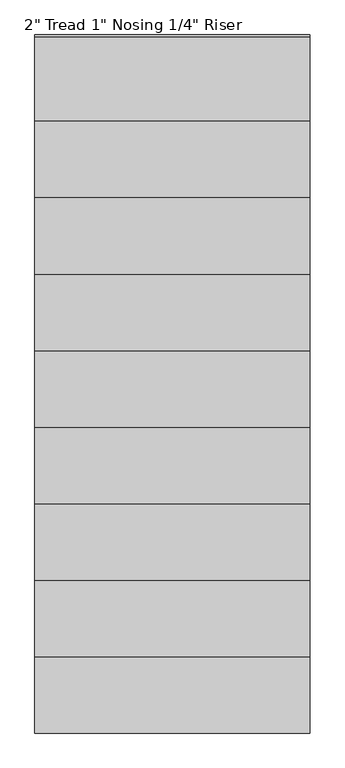
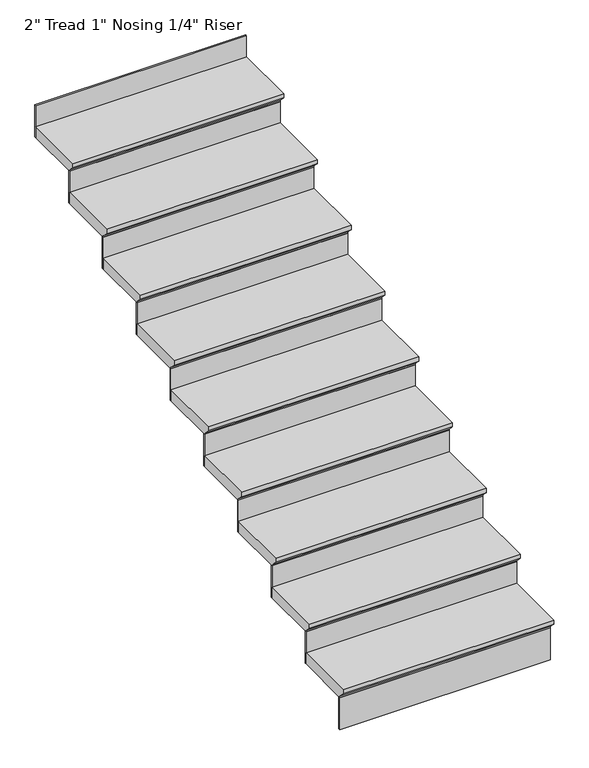
"""IFC4 building model written with IfcOpenShell, lengths in millimetres: stair flight geometry."""

from ifc_helpers import new_model, si_unit, frame, origin, place, context, project, spatial, polyline, outline, extrude, source, transform, mapped, element, save


def stair_flight_6c6ce143(model_context):
    return source(origin(), model_context, "Body", "SweptSolid", [
        extrude(outline(polyline([(-6527.0593836, 11170.7107431), (-6247.6593836, 11170.7107431), (-6247.6593836, 11119.9107431), (-6501.6593836, 11119.9107431), (-6501.6593836, 11126.2607431), (-6527.0593836, 11151.6607431), (-6527.0593836, 11170.7107431)])), frame((-5280.3137331, 0.0, 0.0), z_axis=(1.0, 0.0, 0.0), x_axis=(0.0, 1.0, 0.0)), (0.0, 0.0, 1.0), 914.4),
        extrude(outline(polyline([(-4365.9137331, -6495.3093836), (-4365.9137331, -6501.6593836), (-5280.3137331, -6501.6593836), (-5280.3137331, -6495.3093836), (-4365.9137331, -6495.3093836)])), frame((0.0, 0.0, 10972.0618174), z_axis=(0.0, 0.0, 1.0), x_axis=(1.0, 0.0, 0.0)), (0.0, 0.0, 1.0), 147.8489257),
        extrude(outline(polyline([(-4365.9137331, -6241.3093836), (-4365.9137331, -6247.6593836), (-5280.3137331, -6247.6593836), (-5280.3137331, -6241.3093836), (-4365.9137331, -6241.3093836)])), frame((0.0, 0.0, 11119.9107431), z_axis=(0.0, 0.0, 1.0), x_axis=(1.0, 0.0, 0.0)), (0.0, 0.0, 1.0), 147.8489257),
        extrude(outline(polyline([(-6273.0593836, 11318.5596688), (-5993.6593836, 11318.5596688), (-5993.6593836, 11267.7596688), (-6247.6593836, 11267.7596688), (-6247.6593836, 11274.1096688), (-6273.0593836, 11299.5096688), (-6273.0593836, 11318.5596688)])), frame((-5280.3137331, 0.0, 0.0), z_axis=(1.0, 0.0, 0.0), x_axis=(0.0, 1.0, 0.0)), (0.0, 0.0, 1.0), 914.4),
        extrude(outline(polyline([(-4365.9137331, -5987.3093836), (-4365.9137331, -5993.6593836), (-5280.3137331, -5993.6593836), (-5280.3137331, -5987.3093836), (-4365.9137331, -5987.3093836)])), frame((0.0, 0.0, 11267.7596688), z_axis=(0.0, 0.0, 1.0), x_axis=(1.0, 0.0, 0.0)), (0.0, 0.0, 1.0), 147.8489257),
        extrude(outline(polyline([(-6019.0593836, 11466.4085944), (-5739.6593836, 11466.4085944), (-5739.6593836, 11415.6085944), (-5993.6593836, 11415.6085944), (-5993.6593836, 11421.9585944), (-6019.0593836, 11447.3585944), (-6019.0593836, 11466.4085944)])), frame((-5280.3137331, 0.0, 0.0), z_axis=(1.0, 0.0, 0.0), x_axis=(0.0, 1.0, 0.0)), (0.0, 0.0, 1.0), 914.4),
        extrude(outline(polyline([(-4365.9137331, -5733.3093836), (-4365.9137331, -5739.6593836), (-5280.3137331, -5739.6593836), (-5280.3137331, -5733.3093836), (-4365.9137331, -5733.3093836)])), frame((0.0, 0.0, 11415.6085944), z_axis=(0.0, 0.0, 1.0), x_axis=(1.0, 0.0, 0.0)), (0.0, 0.0, 1.0), 147.8489257),
        extrude(outline(polyline([(-5765.0593836, 11614.2575201), (-5485.6593836, 11614.2575201), (-5485.6593836, 11563.4575201), (-5739.6593836, 11563.4575201), (-5739.6593836, 11569.8075201), (-5765.0593836, 11595.2075201), (-5765.0593836, 11614.2575201)])), frame((-5280.3137331, 0.0, 0.0), z_axis=(1.0, 0.0, 0.0), x_axis=(0.0, 1.0, 0.0)), (0.0, 0.0, 1.0), 914.4),
        extrude(outline(polyline([(-4365.9137331, -5479.3093836), (-4365.9137331, -5485.6593836), (-5280.3137331, -5485.6593836), (-5280.3137331, -5479.3093836), (-4365.9137331, -5479.3093836)])), frame((0.0, 0.0, 11563.4575201), z_axis=(0.0, 0.0, 1.0), x_axis=(1.0, 0.0, 0.0)), (0.0, 0.0, 1.0), 147.8489257),
        extrude(outline(polyline([(-5511.0593836, 11762.1064458), (-5231.6593836, 11762.1064458), (-5231.6593836, 11711.3064458), (-5485.6593836, 11711.3064458), (-5485.6593836, 11717.6564458), (-5511.0593836, 11743.0564458), (-5511.0593836, 11762.1064458)])), frame((-5280.3137331, 0.0, 0.0), z_axis=(1.0, 0.0, 0.0), x_axis=(0.0, 1.0, 0.0)), (0.0, 0.0, 1.0), 914.4),
        extrude(outline(polyline([(-4365.9137331, -5225.3093836), (-4365.9137331, -5231.6593836), (-5280.3137331, -5231.6593836), (-5280.3137331, -5225.3093836), (-4365.9137331, -5225.3093836)])), frame((0.0, 0.0, 11711.3064458), z_axis=(0.0, 0.0, 1.0), x_axis=(1.0, 0.0, 0.0)), (0.0, 0.0, 1.0), 147.8489257),
        extrude(outline(polyline([(-5257.0593836, 11909.9553715), (-4977.6593836, 11909.9553715), (-4977.6593836, 11859.1553715), (-5231.6593836, 11859.1553715), (-5231.6593836, 11865.5053715), (-5257.0593836, 11890.9053715), (-5257.0593836, 11909.9553715)])), frame((-5280.3137331, 0.0, 0.0), z_axis=(1.0, 0.0, 0.0), x_axis=(0.0, 1.0, 0.0)), (0.0, 0.0, 1.0), 914.4),
        extrude(outline(polyline([(-4365.9137331, -4971.3093836), (-4365.9137331, -4977.6593836), (-5280.3137331, -4977.6593836), (-5280.3137331, -4971.3093836), (-4365.9137331, -4971.3093836)])), frame((0.0, 0.0, 11859.1553715), z_axis=(0.0, 0.0, 1.0), x_axis=(1.0, 0.0, 0.0)), (0.0, 0.0, 1.0), 147.8489257),
        extrude(outline(polyline([(-5003.0593836, 12057.8042972), (-4723.6593836, 12057.8042972), (-4723.6593836, 12007.0042972), (-4977.6593836, 12007.0042972), (-4977.6593836, 12013.3542972), (-5003.0593836, 12038.7542972), (-5003.0593836, 12057.8042972)])), frame((-5280.3137331, 0.0, 0.0), z_axis=(1.0, 0.0, 0.0), x_axis=(0.0, 1.0, 0.0)), (0.0, 0.0, 1.0), 914.4),
        extrude(outline(polyline([(-4365.9137331, -4717.3093836), (-4365.9137331, -4723.6593836), (-5280.3137331, -4723.6593836), (-5280.3137331, -4717.3093836), (-4365.9137331, -4717.3093836)])), frame((0.0, 0.0, 12007.0042972), z_axis=(0.0, 0.0, 1.0), x_axis=(1.0, 0.0, 0.0)), (0.0, 0.0, 1.0), 147.8489257),
        extrude(outline(polyline([(-4749.0593836, 12205.6532229), (-4469.6593836, 12205.6532229), (-4469.6593836, 12154.8532229), (-4723.6593836, 12154.8532229), (-4723.6593836, 12161.2032229), (-4749.0593836, 12186.6032229), (-4749.0593836, 12205.6532229)])), frame((-5280.3137331, 0.0, 0.0), z_axis=(1.0, 0.0, 0.0), x_axis=(0.0, 1.0, 0.0)), (0.0, 0.0, 1.0), 914.4),
        extrude(outline(polyline([(-4365.9137331, -4463.3093836), (-4365.9137331, -4469.6593836), (-5280.3137331, -4469.6593836), (-5280.3137331, -4463.3093836), (-4365.9137331, -4463.3093836)])), frame((0.0, 0.0, 12154.8532229), z_axis=(0.0, 0.0, 1.0), x_axis=(1.0, 0.0, 0.0)), (0.0, 0.0, 1.0), 147.8489257),
        extrude(outline(polyline([(-4365.9137331, -4209.3093836), (-4365.9137331, -4215.6593836), (-5280.3137331, -4215.6593836), (-5280.3137331, -4209.3093836), (-4365.9137331, -4209.3093836)])), frame((0.0, 0.0, 12302.7021486), z_axis=(0.0, 0.0, 1.0), x_axis=(1.0, 0.0, 0.0)), (0.0, 0.0, 1.0), 147.8489257),
        extrude(outline(polyline([(-4495.0593836, 12353.5021486), (-4215.6593836, 12353.5021486), (-4215.6593836, 12302.7021486), (-4469.6593836, 12302.7021486), (-4469.6593836, 12309.0521486), (-4495.0593836, 12334.4521486), (-4495.0593836, 12353.5021486)])), frame((-5280.3137331, 0.0, 0.0), z_axis=(1.0, 0.0, 0.0), x_axis=(0.0, 1.0, 0.0)), (0.0, 0.0, 1.0), 914.4),
    ])


if __name__ == "__main__":
    model = new_model("IFC4")
    model_context = context("Model", 3, world=origin())
    ifc_project = project(units=[si_unit("LENGTHUNIT", "METRE", prefix="MILLI")], contexts=[model_context])
    site = spatial("IfcSite", under=ifc_project)
    building = spatial("IfcBuilding", under=site)
    placement = place(None, origin())
    stair_flight_shape = stair_flight_6c6ce143(model_context)
    element("IfcStairFlight", 1, ObjectType="2\" Tread 1\" Nosing 1/4\" Riser", at=placement, inside=building, context=model_context, shape_type="MappedRepresentation", body=[
        mapped(stair_flight_shape, transform((0.0, 0.0, 0.0), x_axis=(1.0, 0.0, 0.0), y_axis=(0.0, 1.0, 0.0), z_axis=(0.0, 0.0, 1.0))),
    ])
    save(model, "model.ifc")
